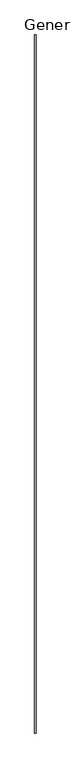
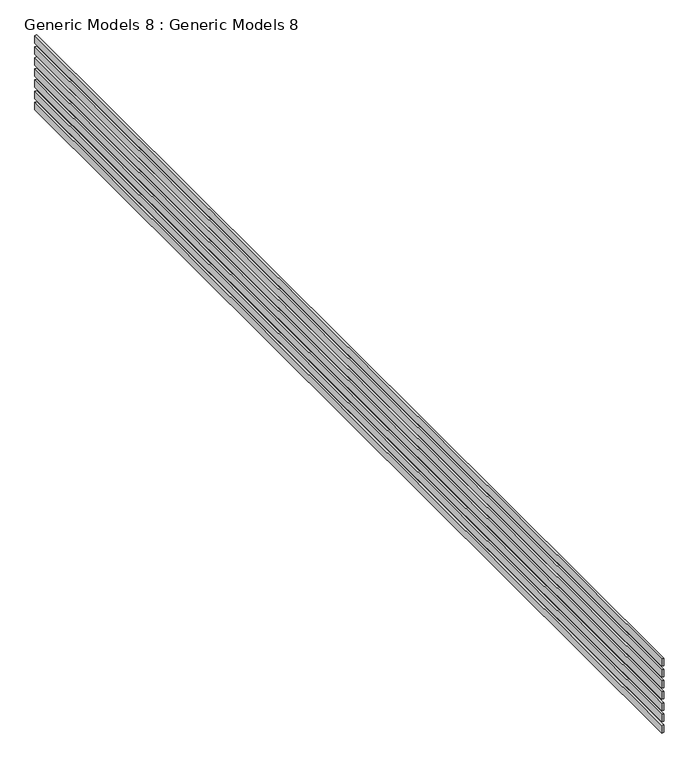
"""IFC4 building model written with IfcOpenShell, lengths in millimetres: proxy geometry, Generic Models 8 : Generic Models 8."""

from ifc_helpers import new_model, si_unit, frame, origin, place, context, project, spatial, polyline, outline, extrude, source, transform, mapped, element, save


def generic_models_8_generic_models_8_cbadd6cc(model_context):
    return source(origin(), model_context, "Body", "SweptSolid", [
        extrude(outline(polyline([(-6319.029089, 10087.4031952), (-6293.629089, 10087.4031952), (-6293.629089, -3876.3468048), (-6319.029089, -3876.3468048), (-6319.029089, 10087.4031952)])), frame((0.0, 0.0, 6877.0852068), z_axis=(0.0, 0.0, 1.0), x_axis=(1.0, 0.0, 0.0)), (0.0, 0.0, 1.0), 101.6),
        extrude(outline(polyline([(-6319.029089, 10087.4031952), (-6293.629089, 10087.4031952), (-6293.629089, -3876.3468048), (-6319.029089, -3876.3468048), (-6319.029089, 10087.4031952)])), frame((0.0, 0.0, 7029.4852068), z_axis=(0.0, 0.0, 1.0), x_axis=(1.0, 0.0, 0.0)), (0.0, 0.0, 1.0), 101.6),
        extrude(outline(polyline([(-6319.029089, 10087.4031952), (-6293.629089, 10087.4031952), (-6293.629089, -3876.3468048), (-6319.029089, -3876.3468048), (-6319.029089, 10087.4031952)])), frame((0.0, 0.0, 7181.8852068), z_axis=(0.0, 0.0, 1.0), x_axis=(1.0, 0.0, 0.0)), (0.0, 0.0, 1.0), 101.6),
        extrude(outline(polyline([(-6319.029089, 10087.4031952), (-6293.629089, 10087.4031952), (-6293.629089, -3876.3468048), (-6319.029089, -3876.3468048), (-6319.029089, 10087.4031952)])), frame((0.0, 0.0, 7334.2852068), z_axis=(0.0, 0.0, 1.0), x_axis=(1.0, 0.0, 0.0)), (0.0, 0.0, 1.0), 101.6),
        extrude(outline(polyline([(-6319.029089, 10087.4031952), (-6293.629089, 10087.4031952), (-6293.629089, -3876.3468048), (-6319.029089, -3876.3468048), (-6319.029089, 10087.4031952)])), frame((0.0, 0.0, 7486.6852068), z_axis=(0.0, 0.0, 1.0), x_axis=(1.0, 0.0, 0.0)), (0.0, 0.0, 1.0), 101.6),
        extrude(outline(polyline([(-6319.029089, 10087.4031952), (-6293.629089, 10087.4031952), (-6293.629089, -3876.3468048), (-6319.029089, -3876.3468048), (-6319.029089, 10087.4031952)])), frame((0.0, 0.0, 7632.7352068), z_axis=(0.0, 0.0, 1.0), x_axis=(1.0, 0.0, 0.0)), (0.0, 0.0, 1.0), 101.6),
        extrude(outline(polyline([(-6319.029089, 10087.4031952), (-6293.629089, 10087.4031952), (-6293.629089, -3876.3468048), (-6319.029089, -3876.3468048), (-6319.029089, 10087.4031952)])), frame((0.0, 0.0, 7785.1352068), z_axis=(0.0, 0.0, 1.0), x_axis=(1.0, 0.0, 0.0)), (0.0, 0.0, 1.0), 101.6),
    ])


if __name__ == "__main__":
    model = new_model("IFC4")
    model_context = context("Model", 3, world=origin())
    ifc_project = project(units=[si_unit("LENGTHUNIT", "METRE", prefix="MILLI")], contexts=[model_context])
    site = spatial("IfcSite", under=ifc_project)
    building = spatial("IfcBuilding", under=site)
    placement = place(None, origin())
    generic_models_8_generic_models_8_shape = generic_models_8_generic_models_8_cbadd6cc(model_context)
    element("IfcBuildingElementProxy", 1, Name="Generic Models 8 : Generic Models 8", ObjectType="Generic Models 8 : Generic Models 8", at=placement, inside=building, context=model_context, shape_type="MappedRepresentation", body=[
        mapped(generic_models_8_generic_models_8_shape, transform((0.0, 0.0, 0.0), x_axis=(1.0, 0.0, 0.0), y_axis=(0.0, 1.0, 0.0), z_axis=(0.0, 0.0, 1.0))),
    ])
    save(model, "model.ifc")

# Revit data of these elements
# Element 1 (IfcBuildingElementProxy, "Generic Models 8 : Generic Models 8")
#   Materials on its faces: "Damp-proofing"
# Materials
#   "Damp-proofing": class "Generic", colour RGB 127 127 127, transparency 0, Description = "Damp-proofing", Cost = 0
